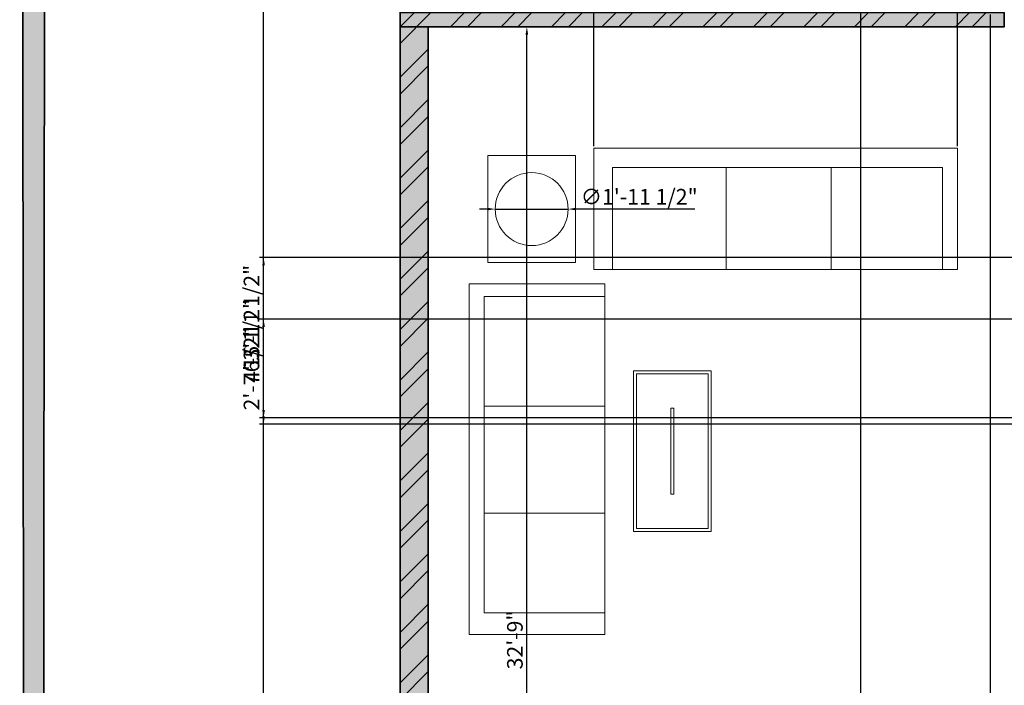
# Model space of a CAD drawing. Units: inches. Extents: x 1804 to 3296, y 909 to 2477.
# Tile 10 of 31: x 1804 to 2119, y 1329 to 1542. Entities that reach past the tile are written whole.
import ezdxf

# ---------------------------------------------------------------- set-up
doc = ezdxf.new("R2010")
doc.units = ezdxf.units.IN
for name, color, linetype, lineweight in [('A-ANNO-DIMS', 2, 'Continuous', 18), ('A-ANNO-TTLB', 156, 'Continuous', 35), ('A-WALL-PATT', 10, 'Continuous', 13), ('FUR', 100, 'Continuous', 18), ('WALL', 10, 'Continuous', 35)]:
    doc.layers.add(name, color=color, linetype=linetype, lineweight=lineweight)
doc.styles.get("Standard").update_dxf_attribs({"font": 'arial.ttf'})
doc.dimstyles.new('ISO-25', dxfattribs={"dimtxt": 5, "dimasz": 2.5, "dimexe": 1.25, "dimexo": 0.625, "dimtad": 1, "dimdec": 0, "dimlunit": 4, "dimtxsty": 'Standard', "dimcen": 2.5, "dimadec": 0, "dimazin": 0, "dimtfac": 1, "dimtdec": 0, "dimtmove": 0, "dimatfit": 3, "dimfxl": 1, "dimarcsym": 0})

# ---------------------------------------------------------------- blocks, each defined once
blk = doc.blocks.new('*D21')
at = {"layer": 'A-ANNO-DIMS', "color": 0, "lineweight": -2, "transparency": 16777216}
for p, q in [((1935.21, 1539.88), (1967.44, 1539.88)), ((1966.19, 1149.57), (1966.19, 1537.38)), ((1935.21, 1147.07), (1967.44, 1147.07))]:
    blk.add_line(p, q, dxfattribs=at)
at = {"layer": 'A-ANNO-DIMS', "color": 0, "lineweight": 100, "transparency": 16777216}
for points in [[(1965.78, 1537.38), (1966.61, 1537.38), (1966.19, 1539.88)], [(1965.78, 1149.57), (1966.61, 1149.57), (1966.19, 1147.07)]]:
    blk.add_solid(points, dxfattribs=at)
at = {"layer": 'Defpoints', "color": 0, "lineweight": 100, "transparency": 16777216}
for p in [(1934.58, 1539.88), (1966.19, 1539.88), (1934.58, 1147.07)]:
    blk.add_point(p, dxfattribs=at)
at = {"layer": 'A-ANNO-DIMS', "color": 0, "transparency": 16777216, "insert": (1963.01, 1343.47), "char_height": 5, "attachment_point": 5, "rotation": 90}
blk.add_mtext('32\'-9"', dxfattribs=at)
blk = doc.blocks.new('*D52')
at = {"layer": 'A-ANNO-DIMS', "color": 0, "lineweight": -2, "transparency": 16777216}
for p, q in [((1924.96, 1830.04), (1880.63, 1830.04)), ((1881.88, 1065.27), (1881.88, 1827.54)), ((1924.96, 1062.77), (1880.63, 1062.77))]:
    blk.add_line(p, q, dxfattribs=at)
at = {"layer": 'A-ANNO-DIMS', "color": 0, "lineweight": 100, "transparency": 16777216}
for points in [[(1881.47, 1827.54), (1882.3, 1827.54), (1881.88, 1830.04)], [(1881.47, 1065.27), (1882.3, 1065.27), (1881.88, 1062.77)]]:
    blk.add_solid(points, dxfattribs=at)
at = {"layer": 'Defpoints', "color": 0, "lineweight": 100, "transparency": 16777216}
for p in [(1881.88, 1830.04), (1925.58, 1830.04), (1925.58, 1062.77)]:
    blk.add_point(p, dxfattribs=at)
at = {"layer": 'A-ANNO-DIMS', "color": 0, "transparency": 16777216, "insert": (1878.67, 1446.4), "char_height": 5, "attachment_point": 5, "rotation": 90}
blk.add_mtext('63\'-11 1/2"', dxfattribs=at)
blk = doc.blocks.new('*D60')
at = {"layer": 'A-ANNO-DIMS', "color": 0, "lineweight": -2, "transparency": 16777216}
for p, q in [((2073.08, 1544.95), (2073.08, 975.89)), ((2114.58, 1543.75), (2114.58, 975.89)), ((2112.08, 977.14), (2075.58, 977.14))]:
    blk.add_line(p, q, dxfattribs=at)
at = {"layer": 'A-ANNO-DIMS', "color": 0, "lineweight": 100, "transparency": 16777216}
for points in [[(2075.58, 977.56), (2075.58, 976.72), (2073.08, 977.14)], [(2112.08, 977.56), (2112.08, 976.72), (2114.58, 977.14)]]:
    blk.add_solid(points, dxfattribs=at)
at = {"layer": 'Defpoints', "color": 0, "lineweight": 100, "transparency": 16777216}
for p in [(2073.08, 1545.58), (2114.58, 1544.38), (2073.08, 977.14)]:
    blk.add_point(p, dxfattribs=at)
at = {"layer": 'A-ANNO-DIMS', "color": 0, "transparency": 16777216, "insert": (2093.83, 980.35), "char_height": 5, "attachment_point": 5}
blk.add_mtext('3\'-5 1/2"', dxfattribs=at)
blk = doc.blocks.new('*D62')
at = {"layer": 'A-ANNO-DIMS', "color": 0, "lineweight": -2, "transparency": 16777216}
for p, q in [((1987.63, 1501.57), (1987.63, 1874.99)), ((1990.13, 1873.74), (2101.57, 1873.74)), ((2104.07, 1501.57), (2104.07, 1874.99))]:
    blk.add_line(p, q, dxfattribs=at)
at = {"layer": 'A-ANNO-DIMS', "color": 0, "lineweight": 100, "transparency": 16777216}
for points in [[(1990.13, 1874.15), (1990.13, 1873.32), (1987.63, 1873.74)], [(2101.57, 1874.15), (2101.57, 1873.32), (2104.07, 1873.74)]]:
    blk.add_solid(points, dxfattribs=at)
at = {"layer": 'Defpoints', "color": 0, "lineweight": 100, "transparency": 16777216}
for p in [(2104.07, 1873.74), (1987.63, 1500.95), (2104.07, 1500.95)]:
    blk.add_point(p, dxfattribs=at)
at = {"layer": 'A-ANNO-DIMS', "color": 0, "transparency": 16777216, "insert": (2045.85, 1876.95), "char_height": 5, "attachment_point": 5}
blk.add_mtext('9\'-8 1/2"', dxfattribs=at)
blk = doc.blocks.new('*D64')
at = {"layer": 'A-ANNO-DIMS', "color": 0, "lineweight": -2, "transparency": 16777216}
for p, q in [((2241.43, 1446.21), (1880.63, 1446.21)), ((1881.88, 1417.08), (1881.88, 1443.71)), ((2241.43, 1414.58), (1880.63, 1414.58))]:
    blk.add_line(p, q, dxfattribs=at)
at = {"layer": 'A-ANNO-DIMS', "color": 0, "lineweight": 100, "transparency": 16777216}
for points in [[(1881.47, 1443.71), (1882.3, 1443.71), (1881.88, 1446.21)], [(1881.47, 1417.08), (1882.3, 1417.08), (1881.88, 1414.58)]]:
    blk.add_solid(points, dxfattribs=at)
at = {"layer": 'Defpoints', "color": 0, "lineweight": 100, "transparency": 16777216}
for p in [(1881.88, 1446.21), (2242.06, 1446.21), (2242.06, 1414.58)]:
    blk.add_point(p, dxfattribs=at)
at = {"layer": 'A-ANNO-DIMS', "color": 0, "transparency": 16777216, "insert": (1878.67, 1430.39), "char_height": 5, "attachment_point": 5, "rotation": 90}
blk.add_mtext('2\'-7 1/2"', dxfattribs=at)
blk = doc.blocks.new('*D66')
at = {"layer": 'A-ANNO-DIMS', "color": 0, "lineweight": -2, "transparency": 16777216}
for p, q in [((2282.03, 1465.94), (1880.63, 1465.94)), ((1881.88, 1415.06), (1881.88, 1463.44)), ((2282.03, 1412.56), (1880.63, 1412.56))]:
    blk.add_line(p, q, dxfattribs=at)
at = {"layer": 'A-ANNO-DIMS', "color": 0, "lineweight": 100, "transparency": 16777216}
for points in [[(1881.47, 1463.44), (1882.3, 1463.44), (1881.88, 1465.94)], [(1881.47, 1415.06), (1882.3, 1415.06), (1881.88, 1412.56)]]:
    blk.add_solid(points, dxfattribs=at)
at = {"layer": 'Defpoints', "color": 0, "lineweight": 100, "transparency": 16777216}
for p in [(1881.88, 1465.94), (2282.65, 1465.94), (2282.65, 1412.56)]:
    blk.add_point(p, dxfattribs=at)
at = {"layer": 'A-ANNO-DIMS', "color": 0, "transparency": 16777216, "insert": (1878.67, 1439.25), "char_height": 5, "attachment_point": 5, "rotation": 90}
blk.add_mtext('4\'-5 1/2"', dxfattribs=at)
blk = doc.blocks.new('*D101')
at = {"layer": 'A-ANNO-DIMS', "color": 0, "lineweight": -2, "transparency": 16777216}
for p, q in [((1953.56, 1481.47), (1951.06, 1481.48)), ((1956.06, 1481.47), (1979.41, 1481.47)), ((2019.93, 1481.46), (1981.91, 1481.47))]:
    blk.add_line(p, q, dxfattribs=at)
at = {"layer": 'A-ANNO-DIMS', "color": 0, "lineweight": 100, "transparency": 16777216}
for points in [[(1953.56, 1481.89), (1953.56, 1481.06), (1956.06, 1481.47)], [(1981.91, 1481.89), (1981.91, 1481.05), (1979.41, 1481.47)]]:
    blk.add_solid(points, dxfattribs=at)
at = {"layer": 'Defpoints', "color": 0, "lineweight": 100, "transparency": 16777216}
for p in [(1956.06, 1481.47), (1979.41, 1481.47)]:
    blk.add_point(p, dxfattribs=at)
at = {"layer": 'A-ANNO-DIMS', "color": 0, "transparency": 16777216, "insert": (2002.17, 1484.78), "char_height": 5, "attachment_point": 5, "rotation": 359.9899}
blk.add_mtext('∅1\'-11 1/2"', dxfattribs=at)

msp = doc.modelspace()

# ---------------------------------------------------------------- hatches: boundary and pattern name
at = {"layer": 'A-ANNO-TTLB'}
h = msp.add_hatch(color=256, dxfattribs=at)
h.dxf.hatch_style = 1
h.paths.add_polyline_path([(3294.53, 2476.54), (1803.79, 2476.54), (1805.43, 909.47), (3296.17, 909.47)])
h.paths.add_polyline_path([(1811, 914.33), (1812.79, 2467.54), (3285.53, 2467.54), (3283.74, 914.33)], flags=16)
h.paths.add_polyline_path([(1925.58, 1062.77), (1925.58, 1138.07), (1925.58, 1539.88), (1925.58, 1793.38), (1925.58, 1830.04), (2325.54, 1830.04), (2325.54, 1793.38), (2325.54, 1586.42), (2325.54, 1138.07), (2325.54, 1062.77)], flags=0)
h.paths.add_polyline_path([(1997.22, 1029.4), (2008.85, 1037.96), (2008.85, 1020.84)], flags=0)
h.paths.add_polyline_path([(1934.58, 1138.07), (1934.58, 1147.07), (2078.77, 1147.07), (2078.77, 1138.07), (2060.94, 1138.07)], flags=0)
h.paths.add_polyline_path([(1944.35, 1138.07), (1944.35, 1147.07), (2056.05, 1147.07), (2056.05, 1138.07)], flags=0)
h.paths.add_polyline_path([(2222.24, 1037.96), (2233.87, 1029.4), (2222.24, 1020.84)], flags=0)
h.paths.add_polyline_path([(2061.94, 1139.07), (2061.94, 1146.07), (2077.77, 1146.07), (2077.77, 1139.07)], flags=0)
h.paths.add_polyline_path([(2149.58, 1138.07), (2149.58, 1269.44), (2158.58, 1269.44), (2158.58, 1326.69), (2149.58, 1326.69), (2149.58, 1340.94), (2139.6, 1340.94), (2139.6, 1434.25), (2149.58, 1434.25), (2149.58, 1447.36), (2158.58, 1447.36), (2158.58, 1423.87), (2158.58, 1408.06), (2198.46, 1408.06), (2198.46, 1412.56), (2282.65, 1412.56), (2282.65, 1465.94), (2316.54, 1465.94), (2316.54, 1590.92), (2192.86, 1590.92), (2192.86, 1595.3), (2291.17, 1595.3), (2291.17, 1590.92), (2316.54, 1590.92), (2316.54, 1784.38), (2300.24, 1784.38), (2300.24, 1757.47), (2268, 1757.47), (2268, 1681.04), (2180.87, 1681.04), (2180.87, 1757.47), (2148.63, 1757.47), (2148.63, 1784.38), (2119.08, 1784.38), (2119.08, 1585.58), (2114.58, 1585.58), (2114.58, 1784.38), (2064.11, 1784.38), (2046.28, 1784.38), (2046.28, 1760.38), (1958.58, 1760.38), (1958.58, 1664.38), (1934.58, 1664.38), (1934.58, 1784.38), (1934.58, 1793.38), (2046.28, 1793.38), (2064.11, 1793.38), (2119.08, 1793.38), (2230.78, 1793.38), (2230.78, 1784.38), (2268, 1784.38), (2300.24, 1784.38), (2316.54, 1784.38), (2316.54, 1590.92), (2316.54, 1373.73), (2316.54, 1138.07)], flags=0)
h.paths.add_polyline_path([(2209.19, 1166.63), (2209.19, 1175.63), (2158.58, 1175.63), (2209.19, 1223.63), (2209.19, 1231.63), (2183.88, 1231.63), (2183.88, 1301.66), (2242.59, 1301.66), (2242.59, 1326.69), (2316.54, 1326.69), (2272.59, 1271.63), (2272.59, 1223.63), (2316.54, 1175.63), (2272.59, 1175.63), (2272.59, 1166.63)], flags=0)
h.paths.add_polyline_path([(1947.77, 1345.22), (1947.77, 1457.48), (1991.2, 1457.48), (1991.2, 1451.7), (1991.2, 1352.18), (1991.2, 1345.22)], flags=0)
h.paths.add_polyline_path([(2209.19, 1271.63), (2262.59, 1271.63), (2262.59, 1311.85), (2272.59, 1301.66), (2272.59, 1271.63), (2269.92, 1269.63), (2270.59, 1269.63), (2270.59, 1225.63), (2211.19, 1225.63), (2211.19, 1269.63), (2211.86, 1269.63)], flags=0)
h.paths.add_polyline_path([(2000.34, 1378.21), (2000.34, 1429.71), (2025.22, 1429.71), (2025.22, 1378.21)], flags=0)
h.paths.add_polyline_path([(2001.34, 1379.21), (2001.34, 1428.71), (2024.22, 1428.71), (2024.22, 1379.21)], flags=0)
h.paths.add_polyline_path([(2012.34, 1390.21), (2012.34, 1417.71), (2013.22, 1417.71), (2013.22, 1390.21)], flags=0)
h.paths.add_polyline_path([(2237.56, 1331.19), (2237.56, 1340.18), (2238.62, 1340.18), (2238.62, 1386.84), (2241.04, 1386.84), (2242.06, 1386.84), (2242.06, 1408.06), (2316.54, 1331.19)], flags=0)
h.paths.add_polyline_path([(1953.73, 1464.35), (1953.73, 1498.59), (1981.74, 1498.59), (1981.74, 1464.35)], flags=0)
h.paths.add_polyline_path([(1987.63, 1462.08), (1987.63, 1500.95), (2104.07, 1500.95), (2104.07, 1462.08), (2099.27, 1462.08), (1993.6, 1462.08)], flags=0)
h.paths.add_polyline_path([(1956.06, 1481.47, -1), (1979.41, 1481.47, -1)], flags=0)
edge = h.paths.add_edge_path(flags=0)
edge.add_ellipse((2299.53, 1438.37), major_axis=(0.31, 21.36), ratio=0.670333, start_angle=0, end_angle=360)
h.paths.add_polyline_path([(2297.39, 1438.37, -1), (2301.67, 1438.37, -1)], flags=0)
h.paths.add_polyline_path([(2591.54, 1163.23), (2591.54, 1179.38), (2591.54, 1379.68), (2591.54, 1395.84), (2734.5, 1395.84), (2734.5, 1379.68), (2734.5, 1179.38), (2734.5, 1163.23)], flags=0)
h.paths.add_polyline_path([(2592.54, 1164.23), (2592.54, 1166.23), (2733.5, 1166.23), (2733.5, 1164.23)], flags=0)
h.paths.add_polyline_path([(2592.54, 1180.38), (2592.54, 1378.68), (2733.5, 1378.68), (2733.5, 1180.38)], flags=0)
h.paths.add_polyline_path([(2593.54, 1181.38), (2593.54, 1377.68), (2732.5, 1377.68), (2732.5, 1181.38)], flags=0)
h.paths.add_polyline_path([(2594.54, 1182.38), (2594.54, 1376.68), (2731.5, 1376.68), (2731.5, 1182.38)], flags=0)
h.paths.add_polyline_path([(1936.95, 1697.46), (1936.95, 1736.46), (1955.41, 1736.46), (1955.41, 1697.46)], flags=0)
h.paths.add_polyline_path([(1938.48, 1718.36), (1938.48, 1734.92), (1953.65, 1734.92), (1953.65, 1718.36)], flags=0)
h.paths.add_polyline_path([(1944.75, 1726.64, -1), (1947.37, 1726.64, -1)], flags=0)
h.paths.add_polyline_path([(2592.54, 1394.84), (2733.5, 1394.84), (2733.5, 1392.84), (2592.54, 1392.84)], flags=0)
h.paths.add_polyline_path([(1976.61, 1762.5), (1976.61, 1781.44), (2012.79, 1781.44), (2012.79, 1762.5)], flags=0)
h.paths.add_polyline_path([(1979.57, 1771.97, -1), (1991.39, 1771.97, -1)], flags=0)
h.paths.add_polyline_path([(1995.36, 1771.97, -1), (2007.18, 1771.97, -1)], flags=0)
h.paths.add_polyline_path([(2251.51, 1744.53), (2268, 1730.05), (2251.51, 1730.05)], flags=0)
h.paths.add_polyline_path([(2047.28, 1785.38), (2047.28, 1792.38), (2063.11, 1792.38), (2063.11, 1785.38)], flags=0)
h.paths.add_polyline_path([(2155.08, 1770.92, -1), (2174.42, 1770.92, -1)], flags=0)
h.paths.add_polyline_path([(2188.59, 1758.27), (2188.59, 1772.81), (2222.3, 1772.81), (2222.3, 1758.27)], flags=0)
h.paths.add_polyline_path([(2223.97, 1758.27), (2223.97, 1772.81), (2257.68, 1772.81), (2257.68, 1758.27)], flags=0)
h.paths.add_polyline_path([(2274.45, 1770.92, -1), (2293.8, 1770.92, -1)], flags=0)
h.paths.add_polyline_path([(2591.54, 1582.09), (2591.54, 1782.39), (2734.5, 1782.39), (2734.5, 1582.09)], flags=0)
h.paths.add_polyline_path([(2592.54, 1583.09), (2592.54, 1781.39), (2733.5, 1781.39), (2733.5, 1583.09)], flags=0)
h.paths.add_polyline_path([(2593.54, 1584.09), (2593.54, 1780.39), (2732.5, 1780.39), (2732.5, 1584.09)], flags=0)
h.paths.add_polyline_path([(2594.54, 1585.09), (2594.54, 1779.39), (2731.5, 1779.39), (2731.5, 1585.09)], flags=0)
h.paths.add_polyline_path([(1922.17, 1978.79), (1922.17, 2295.08), (1922.17, 2296.08), (2115.67, 2296.08), (2115.67, 2384.31), (2115.67, 2385.31), (2322.12, 2385.31), (2323.12, 2385.31), (2323.12, 1979.79), (2323.12, 1978.79), (1923.17, 1978.79)], flags=0)
h.paths.add_polyline_path([(1922.17, 1978.79), (1922.17, 2051.31), (1922.17, 2214.86), (1922.17, 2296.08), (2115.67, 2296.08), (2115.67, 2385.31), (2323.12, 2385.31), (2323.12, 2280.42), (2323.12, 1978.79), (2115.67, 1978.79)], flags=0)
h.paths.add_polyline_path([(1923.17, 1979.79), (1923.17, 2050.31), (2115.67, 2050.31), (2115.67, 2051.31), (1923.17, 2051.31), (1923.17, 2213.86), (1923.17, 2214.86), (1923.17, 2295.08), (1990.02, 2295.08), (1990.02, 2214.86), (1991.02, 2214.86), (1991.02, 2295.08), (2115.67, 2295.08), (2115.67, 1979.79), (2116.67, 1979.79), (2116.67, 2304.18), (2116.67, 2384.31), (2322.12, 2384.31), (2322.12, 2280.42), (2322.12, 1979.79), (2115.67, 1979.79)], flags=0)
h.paths.add_polyline_path([(2972.46, 1192.5), (2972.46, 1196.92), (2995.47, 1196.92), (2995.47, 1255.47), (2995.09, 1255.47), (2987.42, 1249.39), (2980.08, 1255.47), (2978.05, 1255.47), (2978.05, 1257.24), (2995.47, 1257.24), (2995.47, 1261.58), (3015.37, 1261.58), (3015.37, 1333.28), (3015.37, 1414.4), (3032.82, 1414.4), (3032.82, 1333.28), (3032.82, 1261.58), (3052.66, 1261.58), (3052.66, 1255.47), (3079.86, 1255.47), (3078.72, 1254.57), (3081.47, 1252.29), (3078.56, 1249.99), (3075.81, 1252.26), (3072.57, 1249.69), (3070.36, 1251.52), (3067.67, 1249.39), (3060.34, 1255.47), (3052.66, 1255.47), (3052.66, 1196.92), (3054.58, 1196.92), (3074, 1196.92), (3074, 1192.5), (3052.66, 1192.5), (2995.47, 1192.5)], flags=0)
h.paths.add_polyline_path([(2490.75, 1979.27), (2490.75, 1980.27), (2596.87, 1980.27), (2596.87, 2051.8), (2596.87, 2052.8), (2596.87, 2216.35), (2596.87, 2297.57), (2717.32, 2297.57), (2710.57, 2305.62), (2724.07, 2305.62), (2717.32, 2297.57), (2782.37, 2297.57), (2782.37, 2395.8), (3006.82, 2395.8), (3006.82, 1981.27), (3093.73, 1981.27), (3093.73, 1980.27), (3047.51, 1980.27), (3046.37, 1979.37), (3049.11, 1977.1), (3046.2, 1974.79), (3043.46, 1977.07), (3040.21, 1974.49), (3038, 1976.32), (3035.32, 1974.2), (3027.98, 1980.27), (2871.83, 1980.27), (2871.83, 1981.27), (2791.37, 1981.27), (2791.37, 2050.8), (2597.87, 2050.8), (2597.87, 1980.27), (2597.87, 1979.27), (2546.27, 1979.27), (2545.12, 1978.37), (2547.87, 1976.1), (2544.96, 1973.79), (2542.22, 1976.07), (2538.97, 1973.49), (2536.76, 1975.32), (2534.07, 1973.2), (2526.74, 1979.27)], flags=0)
h.paths.add_polyline_path([(2597.87, 2051.8), (2606.87, 2051.8), (2606.87, 2258.39), (2597.87, 2258.39), (2597.87, 2296.57), (2606.87, 2296.57), (2606.87, 2262.39), (2782.37, 2262.39), (2782.37, 2296.57), (2790.37, 2296.57), (2790.37, 2262.39), (2791.37, 2262.39), (2791.37, 2305.67), (2791.37, 2385.8), (2996.82, 2385.8), (2996.82, 2339.85), (3006.82, 2339.85), (3006.82, 2250.12), (2997.82, 2250.12), (2997.82, 1981.27), (2996.82, 1981.27), (2872.83, 1981.27), (2872.83, 1991.8), (2871.83, 1991.8), (2871.83, 2050.8), (2790.37, 2050.8), (2597.87, 2050.8)], flags=0)
h.paths.add_polyline_path([(2179.93, 2153.92), (2179.93, 2353.97), (2259.98, 2353.97), (2259.98, 2153.92)], flags=0)
h.paths.add_polyline_path([(2180.93, 2154.92), (2180.93, 2352.97), (2258.98, 2352.97), (2258.98, 2154.92)], flags=0)
h.paths.add_polyline_path([(2960.87, 1608.49), (2960.87, 1753.62), (3070.9, 1753.62), (3070.9, 1608.49)], flags=0)
h.paths.add_polyline_path([(2961.87, 1609.49), (2961.87, 1752.62), (3069.9, 1752.62), (3069.9, 1609.49)], flags=0)
h.paths.add_polyline_path([(2962.87, 1610.49), (2962.87, 1751.62), (3068.9, 1751.62), (3068.9, 1610.49)], flags=0)
h.paths.add_polyline_path([(2963.87, 1611.49), (2963.87, 1750.62), (3067.9, 1750.62), (3067.9, 1611.49)], flags=0)
h.paths.add_polyline_path([(2782.37, 2051.8), (2782.37, 2216.32), (2791.37, 2216.32), (2791.37, 2051.8), (2872.83, 2051.8), (2872.83, 2068.56), (2884.67, 2068.56), (2884.67, 2085.33), (2896.51, 2085.33), (2896.51, 2102.09), (2908.36, 2102.09), (2908.36, 2118.85), (2920.2, 2118.85), (2920.2, 2135.62), (2932.05, 2135.62), (2932.05, 2145.3), (2925.08, 2145.3), (2925.08, 2203.2), (2996.82, 2203.2), (2996.82, 2145.3), (2953.82, 2145.3), (2872.83, 2051.8), (2790.37, 2051.8)], flags=0)
h.paths.add_polyline_path([(2717.32, 2238.65), (2710.57, 2246.7), (2724.07, 2246.7)], flags=0)
h.paths.add_polyline_path([(2003.09, 1122.79), (2017.16, 1122.79), (2017.16, 1138.74), (2003.09, 1138.74)], flags=8)
h.paths.add_polyline_path([(2174.76, 1792.72), (2188.83, 1792.72), (2188.83, 1808.66), (2174.76, 1808.66)], flags=8)
h.paths.add_polyline_path([(1987.95, 1792.51), (2002.02, 1792.51), (2002.02, 1808.45), (1987.95, 1808.45)], flags=8)
h.paths.add_polyline_path([(2148.79, 1289.26), (2160.46, 1289.26), (2160.46, 1305.2), (2148.79, 1305.2)], flags=8)
h.paths.add_polyline_path([(2115.36, 1133.57), (2127.04, 1133.57), (2127.04, 1149.51), (2115.36, 1149.51)], flags=8)
h.paths.add_polyline_path([(2237.58, 1421.48), (2249.25, 1421.48), (2249.25, 1437.43), (2237.58, 1437.43)], flags=8)
h.paths.add_polyline_path([(2134.99, 1584.32), (2146.66, 1584.32), (2146.66, 1600.26), (2134.99, 1600.26)], flags=8)
h.paths.add_polyline_path([(2101.95, 1557.31), (2113.62, 1557.31), (2113.62, 1573.25), (2101.95, 1573.25)], flags=8)
h.paths.add_polyline_path([(2937.85, 1156.77), (3120.41, 1156.77), (3120.41, 1185.72), (2937.85, 1185.72)], flags=8)
h.paths.add_polyline_path([(2980.71, 1786.71), (3050.06, 1786.71), (3050.06, 1802.66), (2980.71, 1802.66)], flags=8)
h.paths.add_polyline_path([(2869.28, 1661.96), (2938.62, 1661.96), (2938.62, 1690.8), (2869.28, 1690.8)], flags=8)
h.paths.add_polyline_path([(3092.27, 1674.86), (3161.62, 1674.86), (3161.62, 1690.8), (3092.27, 1690.8)], flags=8)
h.paths.add_polyline_path([(2980.71, 1674.86), (3050.06, 1674.86), (3050.06, 1690.8), (2980.71, 1690.8)], flags=8)
h.paths.add_polyline_path([(2649.07, 1678.23), (2674.53, 1678.23), (2674.53, 1714.76), (2649.07, 1714.76)], flags=8)
h.paths.add_polyline_path([(2530.84, 1981.63), (2549.13, 1981.63), (2549.13, 1997.57), (2530.84, 1997.57)], flags=8)
h.paths.add_polyline_path([(3031.29, 1981.77), (3049.58, 1981.77), (3049.58, 1997.71), (3031.29, 1997.71)], flags=8)
h.paths.add_polyline_path([(2715.38, 1911.9), (2851.54, 1911.9), (2851.54, 1940.85), (2715.38, 1940.85)], flags=8)
h.paths.add_polyline_path([(2015.23, 1927.36), (2205.42, 1927.36), (2205.42, 1956.3), (2015.23, 1956.3)], flags=8)
h.paths.add_polyline_path([(2671.84, 2057.84), (2702.75, 2057.84), (2702.75, 2073.79), (2671.84, 2073.79)], flags=8)
h.paths.add_polyline_path([(2678.5, 2316.52), (2765.26, 2316.52), (2765.26, 2332.46), (2678.5, 2332.46)], flags=8)
h.paths.add_polyline_path([(2678.48, 2271.96), (2736.41, 2271.96), (2736.41, 2287.9), (2678.48, 2287.9)], flags=8)
h.paths.add_polyline_path([(2019.2, 972.79), (2243.21, 972.79), (2243.21, 1001.74), (2019.2, 1001.74)], flags=8)
h.paths.add_polyline_path([(2097.06, 1021.56), (2132.16, 1021.56), (2132.16, 1037.51), (2097.06, 1037.51)], flags=8)
h.paths.add_polyline_path([(2182.47, 1360.48), (2207.35, 1360.48), (2207.35, 1376.42), (2182.47, 1376.42)], flags=8)
h.paths.add_polyline_path([(2261.12, 1361.77), (2295.01, 1361.77), (2295.01, 1377.71), (2261.12, 1377.71)], flags=8)
h.paths.add_polyline_path([(2245.75, 1511.51), (2278.44, 1511.51), (2278.44, 1527.46), (2245.75, 1527.46)], flags=8)
h.paths.add_polyline_path([(1991.16, 1296.29), (2060.51, 1296.29), (2060.51, 1312.23), (1991.16, 1312.23)], flags=8)
h.paths.add_polyline_path([(2187, 1651.35), (2246.71, 1651.35), (2246.71, 1667.29), (2187, 1667.29)], flags=8)
h.paths.add_polyline_path([(1976.49, 1684.81), (2068.63, 1684.81), (2068.63, 1700.76), (1976.49, 1700.76)], flags=8)
at = {"layer": 'A-WALL-PATT'}
h = msp.add_hatch(color=256, dxfattribs=at)
h.dxf.hatch_style = 1
h.paths.add_polyline_path([(2119.08, 1544.38), (1925.58, 1544.38), (1925.58, 1539.88), (2119.08, 1539.88)])
h.paths.add_polyline_path([(2119.08, 1545.58), (2114.58, 1545.58), (2114.58, 1544.38), (2119.08, 1544.38)])
h.paths.add_polyline_path([(1965.87, 1658.79), (1965.87, 1679.09), (1955.57, 1679.09), (1955.57, 1658.79)], flags=9)
h.paths.add_polyline_path([(2293.18, 1677.29), (2293.18, 1697.58), (2282.88, 1697.58), (2282.88, 1677.29)], flags=9)
h.paths.add_polyline_path([(2271.13, 1545.23), (2287.53, 1545.23), (2287.53, 1555.53), (2271.13, 1555.53)], flags=9)
h.paths.add_polyline_path([(2303.26, 1488.52), (2303.26, 1508.82), (2292.95, 1508.82), (2292.95, 1488.52)], flags=9)
h.paths.add_polyline_path([(2271.13, 1393.15), (2287.53, 1393.15), (2287.53, 1403.45), (2271.13, 1403.45)], flags=9)
h.paths.add_polyline_path([(2306.48, 1361.45), (2306.48, 1377.86), (2296.18, 1377.86), (2296.18, 1361.45)], flags=9)
h.paths.add_polyline_path([(2174.54, 1361.45), (2174.54, 1377.86), (2164.23, 1377.86), (2164.23, 1361.45)], flags=9)
h.paths.add_polyline_path([(1968.21, 1333.34), (1968.21, 1353.64), (1957.91, 1353.64), (1957.91, 1333.34)], flags=9)
h.paths.add_polyline_path([(2003.09, 1122.79), (2017.16, 1122.79), (2017.16, 1138.74), (2003.09, 1138.74)], flags=9)
h.paths.add_polyline_path([(2174.76, 1792.72), (2188.83, 1792.72), (2188.83, 1808.66), (2174.76, 1808.66)], flags=9)
h.paths.add_polyline_path([(1987.95, 1792.51), (2002.02, 1792.51), (2002.02, 1808.45), (1987.95, 1808.45)], flags=9)
h.paths.add_polyline_path([(2148.79, 1289.26), (2160.46, 1289.26), (2160.46, 1305.2), (2148.79, 1305.2)], flags=9)
h.paths.add_polyline_path([(2115.36, 1133.57), (2127.04, 1133.57), (2127.04, 1149.51), (2115.36, 1149.51)], flags=9)
h.paths.add_polyline_path([(2237.58, 1421.48), (2249.25, 1421.48), (2249.25, 1437.43), (2237.58, 1437.43)], flags=9)
h.paths.add_polyline_path([(2134.99, 1584.32), (2146.66, 1584.32), (2146.66, 1600.26), (2134.99, 1600.26)], flags=9)
h.paths.add_polyline_path([(2101.95, 1557.31), (2113.62, 1557.31), (2113.62, 1573.25), (2101.95, 1573.25)], flags=9)
h.paths.add_polyline_path([(2937.85, 1156.77), (3120.41, 1156.77), (3120.41, 1185.72), (2937.85, 1185.72)], flags=9)
h.paths.add_polyline_path([(2980.71, 1786.71), (3050.06, 1786.71), (3050.06, 1802.66), (2980.71, 1802.66)], flags=9)
h.paths.add_polyline_path([(2869.28, 1661.96), (2938.62, 1661.96), (2938.62, 1690.8), (2869.28, 1690.8)], flags=9)
h.paths.add_polyline_path([(3092.27, 1674.86), (3161.62, 1674.86), (3161.62, 1690.8), (3092.27, 1690.8)], flags=9)
h.paths.add_polyline_path([(2980.71, 1674.86), (3050.06, 1674.86), (3050.06, 1690.8), (2980.71, 1690.8)], flags=9)
h.paths.add_polyline_path([(2649.07, 1678.23), (2674.53, 1678.23), (2674.53, 1714.76), (2649.07, 1714.76)], flags=9)
h.paths.add_polyline_path([(2530.84, 1981.63), (2549.13, 1981.63), (2549.13, 1997.57), (2530.84, 1997.57)], flags=9)
h.paths.add_polyline_path([(3031.29, 1981.77), (3049.58, 1981.77), (3049.58, 1997.71), (3031.29, 1997.71)], flags=9)
h.paths.add_polyline_path([(2715.38, 1911.9), (2851.54, 1911.9), (2851.54, 1940.85), (2715.38, 1940.85)], flags=9)
h.paths.add_polyline_path([(2015.23, 1927.36), (2205.42, 1927.36), (2205.42, 1956.3), (2015.23, 1956.3)], flags=9)
h.paths.add_polyline_path([(2671.84, 2057.84), (2702.75, 2057.84), (2702.75, 2073.79), (2671.84, 2073.79)], flags=9)
h.paths.add_polyline_path([(2678.5, 2316.52), (2765.26, 2316.52), (2765.26, 2332.46), (2678.5, 2332.46)], flags=9)
h.paths.add_polyline_path([(2678.48, 2271.96), (2736.41, 2271.96), (2736.41, 2287.9), (2678.48, 2287.9)], flags=9)
h.paths.add_polyline_path([(2019.2, 972.79), (2243.21, 972.79), (2243.21, 1001.74), (2019.2, 1001.74)], flags=9)
h.paths.add_polyline_path([(2097.06, 1021.56), (2132.16, 1021.56), (2132.16, 1037.51), (2097.06, 1037.51)], flags=9)
h.paths.add_polyline_path([(2182.47, 1360.48), (2207.35, 1360.48), (2207.35, 1376.42), (2182.47, 1376.42)], flags=9)
h.paths.add_polyline_path([(2261.12, 1361.77), (2295.01, 1361.77), (2295.01, 1377.71), (2261.12, 1377.71)], flags=9)
h.paths.add_polyline_path([(2245.75, 1511.51), (2278.44, 1511.51), (2278.44, 1527.46), (2245.75, 1527.46)], flags=9)
h.paths.add_polyline_path([(1991.16, 1296.29), (2060.51, 1296.29), (2060.51, 1312.23), (1991.16, 1312.23)], flags=9)
h.paths.add_polyline_path([(2187, 1651.35), (2246.71, 1651.35), (2246.71, 1667.29), (2187, 1667.29)], flags=9)
h.paths.add_polyline_path([(1976.49, 1684.81), (2068.63, 1684.81), (2068.63, 1700.76), (1976.49, 1700.76)], flags=9)
h = msp.add_hatch(color=256, dxfattribs=at)
h.dxf.hatch_style = 1
h.paths.add_polyline_path([(2158.58, 1275.49), (2155.29, 1275.49), (2149.58, 1275.49), (2149.58, 1269.44), (2158.58, 1269.44)])
h.paths.add_polyline_path([(2158.58, 1326.69), (2149.58, 1326.69), (2149.58, 1319.33), (2155.29, 1319.33), (2158.58, 1319.33)])
h.paths.add_polyline_path([(2158.58, 1402.2), (2158.58, 1423.87), (2158.58, 1447.36), (2149.58, 1447.36), (2149.58, 1423.87), (2149.58, 1340.94), (2149.58, 1326.69), (2158.58, 1326.69), (2158.58, 1354.23)])
h.paths.add_polyline_path([(1965.87, 1658.79), (1965.87, 1679.09), (1955.57, 1679.09), (1955.57, 1658.79)], flags=9)
h.paths.add_polyline_path([(2293.18, 1677.29), (2293.18, 1697.58), (2282.88, 1697.58), (2282.88, 1677.29)], flags=9)
h.paths.add_polyline_path([(2271.13, 1545.23), (2287.53, 1545.23), (2287.53, 1555.53), (2271.13, 1555.53)], flags=9)
h.paths.add_polyline_path([(2303.26, 1488.52), (2303.26, 1508.82), (2292.95, 1508.82), (2292.95, 1488.52)], flags=9)
h.paths.add_polyline_path([(2271.13, 1393.15), (2287.53, 1393.15), (2287.53, 1403.45), (2271.13, 1403.45)], flags=9)
h.paths.add_polyline_path([(2306.48, 1361.45), (2306.48, 1377.86), (2296.18, 1377.86), (2296.18, 1361.45)], flags=9)
h.paths.add_polyline_path([(2189.9, 1340.62), (2206.31, 1340.62), (2206.31, 1350.92), (2189.9, 1350.92)], flags=9)
h.paths.add_polyline_path([(2174.54, 1361.45), (2174.54, 1377.86), (2164.23, 1377.86), (2164.23, 1361.45)], flags=9)
h.paths.add_polyline_path([(2304.24, 1240.8), (2304.24, 1261.09), (2293.94, 1261.09), (2293.94, 1240.8)], flags=9)
h.paths.add_polyline_path([(2227.19, 1188.73), (2247.49, 1188.73), (2247.49, 1199.03), (2227.19, 1199.03)], flags=9)
h.paths.add_polyline_path([(2181.93, 1144.21), (2181.93, 1160.62), (2171.63, 1160.62), (2171.63, 1144.21)], flags=9)
h.paths.add_polyline_path([(1968.21, 1333.34), (1968.21, 1353.64), (1957.91, 1353.64), (1957.91, 1333.34)], flags=9)
h.paths.add_polyline_path([(2029.78, 1203.53), (2053.95, 1203.53), (2053.95, 1213.83), (2029.78, 1213.83)], flags=9)
h.paths.add_polyline_path([(2576.51, 1671.88), (2576.51, 1692.17), (2566.21, 1692.17), (2566.21, 1671.88)], flags=9)
h.paths.add_polyline_path([(2566.99, 1269.67), (2566.99, 1289.96), (2556.68, 1289.96), (2556.68, 1269.67)], flags=9)
h.paths.add_polyline_path([(2581.85, 1269.17), (2581.85, 1289.46), (2571.54, 1289.46), (2571.54, 1269.17)], flags=9)
h.paths.add_polyline_path([(2650.71, 1409.75), (2674.89, 1409.75), (2674.89, 1420.05), (2650.71, 1420.05)], flags=9)
h.paths.add_polyline_path([(2003.09, 1122.79), (2017.16, 1122.79), (2017.16, 1138.74), (2003.09, 1138.74)], flags=9)
h.paths.add_polyline_path([(2174.76, 1792.72), (2188.83, 1792.72), (2188.83, 1808.66), (2174.76, 1808.66)], flags=9)
h.paths.add_polyline_path([(1987.95, 1792.51), (2002.02, 1792.51), (2002.02, 1808.45), (1987.95, 1808.45)], flags=9)
h.paths.add_polyline_path([(2148.79, 1289.26), (2160.46, 1289.26), (2160.46, 1305.2), (2148.79, 1305.2)], flags=9)
h.paths.add_polyline_path([(2115.36, 1133.57), (2127.04, 1133.57), (2127.04, 1149.51), (2115.36, 1149.51)], flags=9)
h.paths.add_polyline_path([(2237.58, 1421.48), (2249.25, 1421.48), (2249.25, 1437.43), (2237.58, 1437.43)], flags=9)
h.paths.add_polyline_path([(2134.99, 1584.32), (2146.66, 1584.32), (2146.66, 1600.26), (2134.99, 1600.26)], flags=9)
h.paths.add_polyline_path([(2101.95, 1557.31), (2113.62, 1557.31), (2113.62, 1573.25), (2101.95, 1573.25)], flags=9)
h.paths.add_polyline_path([(2937.85, 1156.77), (3120.41, 1156.77), (3120.41, 1185.72), (2937.85, 1185.72)], flags=9)
h.paths.add_polyline_path([(2980.71, 1786.71), (3050.06, 1786.71), (3050.06, 1802.66), (2980.71, 1802.66)], flags=9)
h.paths.add_polyline_path([(2869.28, 1661.96), (2938.62, 1661.96), (2938.62, 1690.8), (2869.28, 1690.8)], flags=9)
h.paths.add_polyline_path([(3092.27, 1674.86), (3161.62, 1674.86), (3161.62, 1690.8), (3092.27, 1690.8)], flags=9)
h.paths.add_polyline_path([(2980.71, 1674.86), (3050.06, 1674.86), (3050.06, 1690.8), (2980.71, 1690.8)], flags=9)
h.paths.add_polyline_path([(2649.07, 1678.23), (2674.53, 1678.23), (2674.53, 1714.76), (2649.07, 1714.76)], flags=9)
h.paths.add_polyline_path([(2530.84, 1981.63), (2549.13, 1981.63), (2549.13, 1997.57), (2530.84, 1997.57)], flags=9)
h.paths.add_polyline_path([(3031.29, 1981.77), (3049.58, 1981.77), (3049.58, 1997.71), (3031.29, 1997.71)], flags=9)
h.paths.add_polyline_path([(2715.38, 1911.9), (2851.54, 1911.9), (2851.54, 1940.85), (2715.38, 1940.85)], flags=9)
h.paths.add_polyline_path([(2015.23, 1927.36), (2205.42, 1927.36), (2205.42, 1956.3), (2015.23, 1956.3)], flags=9)
h.paths.add_polyline_path([(2671.84, 2057.84), (2702.75, 2057.84), (2702.75, 2073.79), (2671.84, 2073.79)], flags=9)
h.paths.add_polyline_path([(2678.5, 2316.52), (2765.26, 2316.52), (2765.26, 2332.46), (2678.5, 2332.46)], flags=9)
h.paths.add_polyline_path([(2678.48, 2271.96), (2736.41, 2271.96), (2736.41, 2287.9), (2678.48, 2287.9)], flags=9)
h.paths.add_polyline_path([(2019.2, 972.79), (2243.21, 972.79), (2243.21, 1001.74), (2019.2, 1001.74)], flags=9)
h.paths.add_polyline_path([(2097.06, 1021.56), (2132.16, 1021.56), (2132.16, 1037.51), (2097.06, 1037.51)], flags=9)
h.paths.add_polyline_path([(2182.47, 1360.48), (2207.35, 1360.48), (2207.35, 1376.42), (2182.47, 1376.42)], flags=9)
h.paths.add_polyline_path([(2261.12, 1361.77), (2295.01, 1361.77), (2295.01, 1377.71), (2261.12, 1377.71)], flags=9)
h.paths.add_polyline_path([(2245.75, 1511.51), (2278.44, 1511.51), (2278.44, 1527.46), (2245.75, 1527.46)], flags=9)
h.paths.add_polyline_path([(1991.16, 1296.29), (2060.51, 1296.29), (2060.51, 1312.23), (1991.16, 1312.23)], flags=9)
h.paths.add_polyline_path([(2187, 1651.35), (2246.71, 1651.35), (2246.71, 1667.29), (2187, 1667.29)], flags=9)
h.paths.add_polyline_path([(1976.49, 1684.81), (2068.63, 1684.81), (2068.63, 1700.76), (1976.49, 1700.76)], flags=9)
h = msp.add_hatch(dxfattribs=at)
h.set_pattern_fill('ANSI32', color=256, scale=1.2)
h.set_pattern_definition([(45, (0, 196.207), (-8.08223, 8.08223), []), (45, (5.388, 196.207), (-8.08223, 8.08223), [])])
h.paths.add_polyline_path([(1934.58, 1784.38), (1934.58, 1793.38), (1925.58, 1793.38), (1925.58, 1539.88), (2119.08, 1539.88), (2119.08, 1545.58), (2114.58, 1545.58), (2114.58, 1544.38), (1934.58, 1544.38)])
h.paths.add_polyline_path([(2114.58, 1793.38), (2064.11, 1793.38), (2064.11, 1784.38), (2114.58, 1784.38)], flags=17)
h.paths.add_polyline_path([(2325.54, 1793.38), (2230.78, 1793.38), (2230.78, 1784.38), (2268, 1784.38), (2300.24, 1784.38), (2316.54, 1784.38), (2316.54, 1590.92), (2316.54, 1586.42), (2325.54, 1586.42)])
h.paths.add_polyline_path([(1944.35, 1147.07), (1934.58, 1147.07), (1934.58, 1138.07), (1944.35, 1138.07)])
h.paths.add_polyline_path([(2101.21, 1144.07, -0.01877), (2101.32, 1147.07), (2078.77, 1147.07), (2078.77, 1138.07), (2101.21, 1138.07)])
h.paths.add_polyline_path([(1934.58, 1539.88), (1925.58, 1539.88), (1925.58, 1138.07), (1934.58, 1138.07), (1934.58, 1147.07)])
h.paths.add_polyline_path([(2325.54, 1586.42), (2316.54, 1586.42), (2316.54, 1373.73), (2316.54, 1138.07), (2325.54, 1138.07), (2325.54, 1228.97)])
h.paths.add_polyline_path([(2158.58, 1423.87), (2158.58, 1447.36), (2149.58, 1447.36), (2149.58, 1423.87), (2149.58, 1340.94), (2149.58, 1326.69), (2158.58, 1326.69), (2158.58, 1354.23), (2158.58, 1402.2)])
h.paths.add_polyline_path([(2316.54, 1412.56), (2282.65, 1412.56), (2273.09, 1412.56), (2273.09, 1408.06), (2316.54, 1408.06)])
h.paths.add_polyline_path([(2273.09, 1412.56), (2242.06, 1412.56), (2242.06, 1408.06), (2273.09, 1408.06)])
h.paths.add_polyline_path([(2237.56, 1412.56), (2198.46, 1412.56), (2198.46, 1408.06), (2237.56, 1408.06)])
h.paths.add_polyline_path([(2242.06, 1408.06), (2237.56, 1408.06), (2237.56, 1386.84), (2242.06, 1386.84)])
h.paths.add_polyline_path([(2242.06, 1412.56), (2237.56, 1412.56), (2237.56, 1408.06), (2242.06, 1408.06)])
h.paths.add_polyline_path([(2158.58, 1269.44), (2149.58, 1269.44), (2149.58, 1138.07), (2158.58, 1138.07)])
h.paths.add_polyline_path([(2149.58, 1147.07), (2141.21, 1147.07), (2141.21, 1144.07), (2141.21, 1138.07), (2149.58, 1138.07)])
h.paths.add_polyline_path([(2272.59, 1175.63), (2209.19, 1175.63), (2209.19, 1166.63), (2272.59, 1166.63)])
h.paths.add_polyline_path([(2237.56, 1446.21), (2242.06, 1446.21), (2242.06, 1586.42), (2237.56, 1586.42)])
h.paths.add_polyline_path([(2242.06, 1414.58), (2237.56, 1414.58), (2237.56, 1412.56), (2242.06, 1412.56)])
h = msp.add_hatch(color=256, dxfattribs=at)
h.dxf.hatch_style = 1
h.paths.add_polyline_path([(1934.58, 1793.38), (1925.58, 1793.38), (1925.58, 1544.38), (1934.58, 1544.38)])
h.paths.add_polyline_path([(1934.58, 1539.88), (1925.58, 1539.88), (1925.58, 1138.07), (1934.58, 1138.07)])

# ---------------------------------------------------------------- linework, layer by layer
at = {"layer": 'A-ANNO-TTLB'}
for points in [[(1803.79, 2476.54), (3294.53, 2476.54), (3296.17, 909.47), (1805.43, 909.47)], [(1812.79, 2467.54), (3285.53, 2467.54), (3283.74, 914.33), (1811, 914.33)]]:
    msp.add_lwpolyline(points, close=True, dxfattribs=at)
at = {"layer": 'FUR'}
for p, q in [((1987.63, 1462.08), (1987.63, 1500.95)), ((1987.63, 1500.95), (2104.07, 1500.95)), ((2104.07, 1500.95), (2104.07, 1462.08)), ((2030.02, 1494.82), (2030.02, 1462.08)), ((2063.6, 1494.82), (2063.6, 1462.08)), ((1993.6, 1462.08), (1987.63, 1462.08)), ((2099.27, 1462.08), (2104.07, 1462.08)), ((1947.77, 1345.22), (1947.77, 1457.48)), ((1947.77, 1457.48), (1991.2, 1457.48)), ((1991.2, 1457.48), (1991.2, 1451.7)), ((1952.5, 1418.31), (1991.2, 1418.31)), ((1952.5, 1384.04), (1991.2, 1384.04)), ((1991.2, 1352.18), (1991.2, 1345.22)), ((1991.2, 1345.22), (1947.77, 1345.22))]:
    msp.add_line(p, q, dxfattribs=at)
for points in [[(1981.74, 1464.35), (1953.73, 1464.35), (1953.73, 1498.59), (1981.74, 1498.59)], [(1993.6, 1494.82), (2099.27, 1494.82), (2099.27, 1462.08), (1993.6, 1462.08)], [(1952.5, 1352.18), (1991.2, 1352.18), (1991.2, 1453.44), (1952.5, 1453.44)], [(2000.34, 1378.21), (2025.22, 1378.21), (2025.22, 1429.71), (2000.34, 1429.71)], [(2001.34, 1379.21), (2024.22, 1379.21), (2024.22, 1428.71), (2001.34, 1428.71)], [(2012.34, 1390.21), (2013.22, 1390.21), (2013.22, 1417.71), (2012.34, 1417.71)]]:
    msp.add_lwpolyline(points, close=True, dxfattribs=at)
msp.add_circle((1967.74, 1481.47), 11.68, dxfattribs=at)
msp.add_circle((1967.74, 1481.47), 11.68, dxfattribs=at)
at = {"layer": 'WALL'}
for p, q in [((1925.58, 1539.88), (1925.58, 1793.38)), ((2119.08, 1539.88), (1925.58, 1539.88)), ((1925.58, 1539.88), (1925.58, 1138.07)), ((1934.58, 1539.88), (1934.58, 1138.07))]:
    msp.add_line(p, q, dxfattribs=at)
for points in [[(1925.58, 1539.88), (2119.08, 1539.88), (2119.08, 1544.38), (1925.58, 1544.38)], [(1925.58, 1138.07), (1934.58, 1138.07), (1934.58, 1539.88), (1925.58, 1539.88)]]:
    msp.add_lwpolyline(points, close=True, dxfattribs=at)

# ---------------------------------------------------------------- dimensions: what is measured, and where the dimension line sits
at = {"layer": 'A-ANNO-DIMS'}
for base, p1, p2, picture, middle in [((2104.07, 1873.74), (1987.63, 1500.95), (2104.07, 1500.95), '*D62', (2045.85, 1876.95)), ((2073.08, 977.14), (2114.58, 1544.38), (2073.08, 1545.58), '*D60', (2093.83, 980.35))]:
    dim = msp.add_linear_dim(base=base, p1=p1, p2=p2, dimstyle='ISO-25', override={"dimdec": 1, "dimlfac": 1, "dimrnd": 0, "dimzin": 1, "dimdsep": 46, "dimlunit": 4, "dimfrac": 2}, dxfattribs=at)
    dim.commit()
    dim.dimension.update_dxf_attribs({"geometry": picture, "text_midpoint": middle})
for base, p1, p2, override, picture, middle in [((1881.88, 1830.04), (1925.58, 1062.77), (1925.58, 1830.04), {"dimdec": 1, "dimlfac": 1, "dimrnd": 0, "dimzin": 1, "dimdsep": 46, "dimlunit": 4, "dimfrac": 2}, '*D52', (1878.67, 1446.4)), ((1966.19, 1539.88), (1934.58, 1147.07), (1934.58, 1539.88), {"dimclrd": 0, "dimclre": 0, "dimclrt": 0}, '*D21', (1963.01, 1343.47)), ((1881.88, 1465.94), (2282.65, 1412.56), (2282.65, 1465.94), {"dimdec": 1, "dimlfac": 1, "dimrnd": 0, "dimzin": 1, "dimdsep": 46, "dimlunit": 4, "dimfrac": 2}, '*D66', (1878.67, 1439.25)), ((1881.88, 1446.21), (2242.06, 1414.58), (2242.06, 1446.21), {"dimdec": 1, "dimlfac": 1, "dimrnd": 0, "dimzin": 1, "dimdsep": 46, "dimlunit": 4, "dimfrac": 2}, '*D64', (1878.67, 1430.39))]:
    dim = msp.add_linear_dim(base=base, p1=p1, p2=p2, angle=90, dimstyle='ISO-25', override=override, dxfattribs=at)
    dim.commit()
    dim.dimension.update_dxf_attribs({"geometry": picture, "text_midpoint": middle})
dim = msp.add_diameter_dim_2p(p1=(1956.0573, 1481.4741), p2=(1979.4132, 1481.47), dimstyle='ISO-25', override={"dimdec": 1, "dimlfac": 1, "dimrnd": 0, "dimzin": 1, "dimdsep": 46, "dimlunit": 4, "dimfrac": 2}, dxfattribs=at)
dim.commit()
dim.dimension.update_dxf_attribs({"geometry": '*D101', "text_midpoint": (2002.1715, 1481.466)})

doc.saveas('drawing.dxf')
